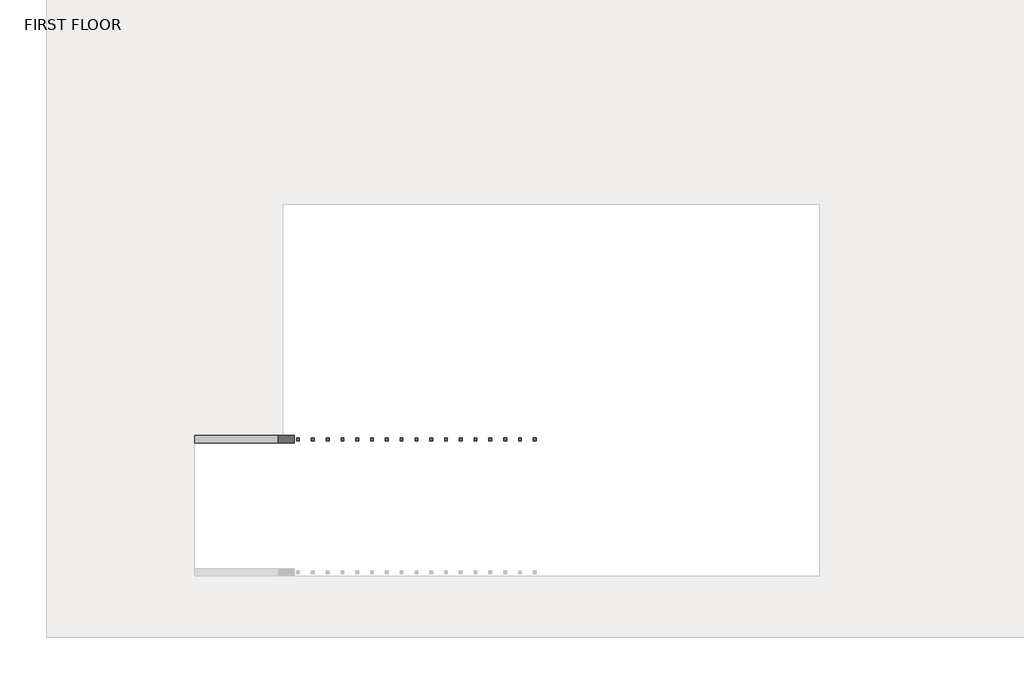
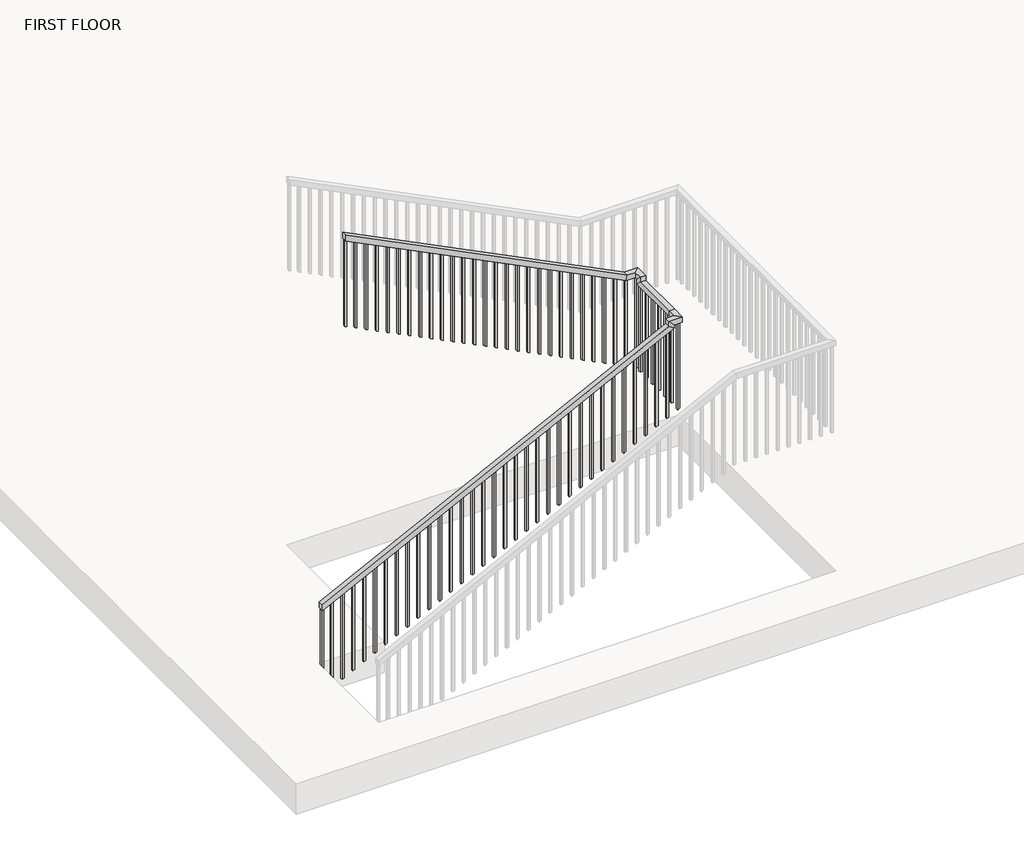
# One storey, part 2 of 2: 1 railing.
"""IFC4 building model written with IfcOpenShell, lengths in millimetres."""

from ifc_helpers import new_model, si_unit, frame, origin, place, context, project, spatial, polyline, outline, extrude, faceted_brep, element, save

model = new_model("IFC4")

# Units and contexts
model_context = context("Model", 3, world=origin())
ifc_project = project(units=[si_unit("LENGTHUNIT", "METRE", prefix="MILLI")], contexts=[model_context])

# Site, building, storey
site = spatial("IfcSite", under=ifc_project)
building = spatial("IfcBuilding", under=site)
storey = spatial("IfcBuildingStorey", under=building, Name="FIRST FLOOR", Elevation=3048.0)

# Railing
placement = place(None, origin())
element("IfcRailing", 1, ObjectType="Handrail - Rectangular", at=placement, inside=storey, context=model_context, shape_type="SolidModel", body=[
    faceted_brep([(-8362.2800418, -4455.7090076, 3962.4), (-8362.2800418, -4455.7090076, 3905.6038734), (-8362.2800418, -4506.5090076, 3905.6038734), (-8362.2800418, -4506.5090076, 3962.4), (-5111.0800418, -4455.7090076, 5588.0), (-5060.2800418, -4455.7090076, 5556.6038734), (-5060.2800418, -4506.5090076, 5556.6038734), (-5111.0800418, -4506.5090076, 5588.0), (-5111.0800418, -4455.7090076, 5638.8), (-5060.2800418, -4455.7090076, 5588.0), (-5060.2800418, -4506.5090076, 5588.0), (-5111.0800418, -4506.5090076, 5638.8), (-5034.8800418, -4455.7090076, 5638.8), (-5034.8800418, -4455.7090076, 5588.0), (-4984.0800418, -4506.5090076, 5588.0), (-4984.0800418, -4506.5090076, 5638.8), (-5034.8800418, -4379.5090076, 5638.8), (-5034.8800418, -4379.5090076, 5588.0), (-4984.0800418, -4379.5090076, 5588.0), (-4984.0800418, -4379.5090076, 5638.8), (-5034.8800418, -3907.7346494, 5638.8), (-5034.8800418, -3856.9346494, 5588.0), (-4984.0800418, -3856.9346494, 5588.0), (-4984.0800418, -3907.7346494, 5638.8), (-5034.8800418, -3907.7346494, 5689.6), (-5034.8800418, -3856.9346494, 5638.8), (-4984.0800418, -3856.9346494, 5638.8), (-4984.0800418, -3907.7346494, 5689.6), (-5034.8800418, -3831.5346494, 5689.6), (-5034.8800418, -3831.5346494, 5638.8), (-4984.0800418, -3780.7346494, 5638.8), (-4984.0800418, -3780.7346494, 5689.6), (-5111.0800418, -3831.5346494, 5689.6), (-5123.072295, -3831.5346494, 5638.8), (-5123.072295, -3780.7346494, 5638.8), (-5111.0800418, -3780.7346494, 5689.6), (-7752.6800418, -3831.5346494, 7010.4), (-7752.6800418, -3780.7346494, 7010.4), (-7752.6800418, -3780.7346494, 6953.6038734), (-7752.6800418, -3831.5346494, 6953.6038734)], [[[0, 1, 2, 3]], [[1, 0, 4, 5]], [[2, 1, 5, 6]], [[3, 2, 6, 7]], [[0, 3, 7, 4]], [[5, 4, 8, 9]], [[6, 5, 9, 10]], [[7, 6, 10, 11]], [[4, 7, 11, 8]], [[9, 8, 12, 13]], [[10, 9, 13, 14]], [[11, 10, 14, 15]], [[8, 11, 15, 12]], [[13, 12, 16, 17]], [[14, 13, 17, 18]], [[15, 14, 18, 19]], [[12, 15, 19, 16]], [[17, 16, 20, 21]], [[18, 17, 21, 22]], [[19, 18, 22, 23]], [[16, 19, 23, 20]], [[21, 20, 24, 25]], [[22, 21, 25, 26]], [[23, 22, 26, 27]], [[20, 23, 27, 24]], [[25, 24, 28, 29]], [[26, 25, 29, 30]], [[27, 26, 30, 31]], [[24, 27, 31, 28]], [[29, 28, 32, 33]], [[30, 29, 33, 34]], [[31, 30, 34, 35]], [[28, 31, 35, 32]], [[36, 37, 38, 39]], [[33, 32, 36, 39]], [[34, 33, 39, 38]], [[35, 34, 38, 37]], [[32, 35, 37, 36]]]),
    extrude(outline(polyline([(6898.0413734, -7641.5550418), (6907.5663734, -7660.6050418), (6049.9625, -7660.6050418), (6040.4375, -7641.5550418), (6898.0413734, -7641.5550418)])), frame((0.0, -3815.6596494, 0.0), z_axis=(0.0, 1.0, 0.0), x_axis=(0.0, 0.0, 1.0)), (0.0, 0.0, 1.0), 19.05),
    extrude(outline(polyline([(6847.2413734, -7539.9550418), (6856.7663734, -7559.0050418), (5999.1625, -7559.0050418), (5989.6375, -7539.9550418), (6847.2413734, -7539.9550418)])), frame((0.0, -3815.6596494, 0.0), z_axis=(0.0, 1.0, 0.0), x_axis=(0.0, 0.0, 1.0)), (0.0, 0.0, 1.0), 19.05),
    extrude(outline(polyline([(6796.4413734, -7438.3550418), (6805.9663734, -7457.4050418), (5948.3625, -7457.4050418), (5938.8375, -7438.3550418), (6796.4413734, -7438.3550418)])), frame((0.0, -3815.6596494, 0.0), z_axis=(0.0, 1.0, 0.0), x_axis=(0.0, 0.0, 1.0)), (0.0, 0.0, 1.0), 19.05),
    extrude(outline(polyline([(6745.6413734, -7336.7550418), (6755.1663734, -7355.8050418), (5897.5625, -7355.8050418), (5888.0375, -7336.7550418), (6745.6413734, -7336.7550418)])), frame((0.0, -3815.6596494, 0.0), z_axis=(0.0, 1.0, 0.0), x_axis=(0.0, 0.0, 1.0)), (0.0, 0.0, 1.0), 19.05),
    extrude(outline(polyline([(6694.8413734, -7235.1550418), (6704.3663734, -7254.2050418), (5846.7625, -7254.2050418), (5837.2375, -7235.1550418), (6694.8413734, -7235.1550418)])), frame((0.0, -3815.6596494, 0.0), z_axis=(0.0, 1.0, 0.0), x_axis=(0.0, 0.0, 1.0)), (0.0, 0.0, 1.0), 19.05),
    extrude(outline(polyline([(6644.0413734, -7133.5550418), (6653.5663734, -7152.6050418), (5795.9625, -7152.6050418), (5786.4375, -7133.5550418), (6644.0413734, -7133.5550418)])), frame((0.0, -3815.6596494, 0.0), z_axis=(0.0, 1.0, 0.0), x_axis=(0.0, 0.0, 1.0)), (0.0, 0.0, 1.0), 19.05),
    extrude(outline(polyline([(6593.2413734, -7031.9550418), (6602.7663734, -7051.0050418), (5745.1625, -7051.0050418), (5735.6375, -7031.9550418), (6593.2413734, -7031.9550418)])), frame((0.0, -3815.6596494, 0.0), z_axis=(0.0, 1.0, 0.0), x_axis=(0.0, 0.0, 1.0)), (0.0, 0.0, 1.0), 19.05),
    extrude(outline(polyline([(6542.4413734, -6930.3550418), (6551.9663734, -6949.4050418), (5694.3625, -6949.4050418), (5684.8375, -6930.3550418), (6542.4413734, -6930.3550418)])), frame((0.0, -3815.6596494, 0.0), z_axis=(0.0, 1.0, 0.0), x_axis=(0.0, 0.0, 1.0)), (0.0, 0.0, 1.0), 19.05),
    extrude(outline(polyline([(6491.6413734, -6828.7550418), (6501.1663734, -6847.8050418), (5643.5625, -6847.8050418), (5634.0375, -6828.7550418), (6491.6413734, -6828.7550418)])), frame((0.0, -3815.6596494, 0.0), z_axis=(0.0, 1.0, 0.0), x_axis=(0.0, 0.0, 1.0)), (0.0, 0.0, 1.0), 19.05),
    extrude(outline(polyline([(6440.8413734, -6727.1550418), (6450.3663734, -6746.2050418), (5592.7625, -6746.2050418), (5583.2375, -6727.1550418), (6440.8413734, -6727.1550418)])), frame((0.0, -3815.6596494, 0.0), z_axis=(0.0, 1.0, 0.0), x_axis=(0.0, 0.0, 1.0)), (0.0, 0.0, 1.0), 19.05),
    extrude(outline(polyline([(6390.0413734, -6625.5550418), (6399.5663734, -6644.6050418), (5541.9625, -6644.6050418), (5532.4375, -6625.5550418), (6390.0413734, -6625.5550418)])), frame((0.0, -3815.6596494, 0.0), z_axis=(0.0, 1.0, 0.0), x_axis=(0.0, 0.0, 1.0)), (0.0, 0.0, 1.0), 19.05),
    extrude(outline(polyline([(6339.2413734, -6523.9550418), (6348.7663734, -6543.0050418), (5491.1625, -6543.0050418), (5481.6375, -6523.9550418), (6339.2413734, -6523.9550418)])), frame((0.0, -3815.6596494, 0.0), z_axis=(0.0, 1.0, 0.0), x_axis=(0.0, 0.0, 1.0)), (0.0, 0.0, 1.0), 19.05),
    extrude(outline(polyline([(6288.4413734, -6422.3550418), (6297.9663734, -6441.4050418), (5440.3625, -6441.4050418), (5430.8375, -6422.3550418), (6288.4413734, -6422.3550418)])), frame((0.0, -3815.6596494, 0.0), z_axis=(0.0, 1.0, 0.0), x_axis=(0.0, 0.0, 1.0)), (0.0, 0.0, 1.0), 19.05),
    extrude(outline(polyline([(6237.6413734, -6320.7550418), (6247.1663734, -6339.8050418), (5389.5625, -6339.8050418), (5380.0375, -6320.7550418), (6237.6413734, -6320.7550418)])), frame((0.0, -3815.6596494, 0.0), z_axis=(0.0, 1.0, 0.0), x_axis=(0.0, 0.0, 1.0)), (0.0, 0.0, 1.0), 19.05),
    extrude(outline(polyline([(6186.8413734, -6219.1550418), (6196.3663734, -6238.2050418), (5338.7625, -6238.2050418), (5329.2375, -6219.1550418), (6186.8413734, -6219.1550418)])), frame((0.0, -3815.6596494, 0.0), z_axis=(0.0, 1.0, 0.0), x_axis=(0.0, 0.0, 1.0)), (0.0, 0.0, 1.0), 19.05),
    extrude(outline(polyline([(6136.0413734, -6117.5550418), (6145.5663734, -6136.6050418), (5287.9625, -6136.6050418), (5278.4375, -6117.5550418), (6136.0413734, -6117.5550418)])), frame((0.0, -3815.6596494, 0.0), z_axis=(0.0, 1.0, 0.0), x_axis=(0.0, 0.0, 1.0)), (0.0, 0.0, 1.0), 19.05),
    extrude(outline(polyline([(6085.2413734, -6015.9550418), (6094.7663734, -6035.0050418), (5237.1625, -6035.0050418), (5227.6375, -6015.9550418), (6085.2413734, -6015.9550418)])), frame((0.0, -3815.6596494, 0.0), z_axis=(0.0, 1.0, 0.0), x_axis=(0.0, 0.0, 1.0)), (0.0, 0.0, 1.0), 19.05),
    extrude(outline(polyline([(6034.4413734, -5914.3550418), (6043.9663734, -5933.4050418), (5186.3625, -5933.4050418), (5176.8375, -5914.3550418), (6034.4413734, -5914.3550418)])), frame((0.0, -3815.6596494, 0.0), z_axis=(0.0, 1.0, 0.0), x_axis=(0.0, 0.0, 1.0)), (0.0, 0.0, 1.0), 19.05),
    extrude(outline(polyline([(5983.6413734, -5812.7550418), (5993.1663734, -5831.8050418), (5135.5625, -5831.8050418), (5126.0375, -5812.7550418), (5983.6413734, -5812.7550418)])), frame((0.0, -3815.6596494, 0.0), z_axis=(0.0, 1.0, 0.0), x_axis=(0.0, 0.0, 1.0)), (0.0, 0.0, 1.0), 19.05),
    extrude(outline(polyline([(5932.8413734, -5711.1550418), (5942.3663734, -5730.2050418), (5084.7625, -5730.2050418), (5075.2375, -5711.1550418), (5932.8413734, -5711.1550418)])), frame((0.0, -3815.6596494, 0.0), z_axis=(0.0, 1.0, 0.0), x_axis=(0.0, 0.0, 1.0)), (0.0, 0.0, 1.0), 19.05),
    extrude(outline(polyline([(5882.0413734, -5609.5550418), (5891.5663734, -5628.6050418), (5033.9625, -5628.6050418), (5024.4375, -5609.5550418), (5882.0413734, -5609.5550418)])), frame((0.0, -3815.6596494, 0.0), z_axis=(0.0, 1.0, 0.0), x_axis=(0.0, 0.0, 1.0)), (0.0, 0.0, 1.0), 19.05),
    extrude(outline(polyline([(5831.2413734, -5507.9550418), (5840.7663734, -5527.0050418), (4983.1625, -5527.0050418), (4973.6375, -5507.9550418), (5831.2413734, -5507.9550418)])), frame((0.0, -3815.6596494, 0.0), z_axis=(0.0, 1.0, 0.0), x_axis=(0.0, 0.0, 1.0)), (0.0, 0.0, 1.0), 19.05),
    extrude(outline(polyline([(5780.4413734, -5406.3550418), (5789.9663734, -5425.4050418), (4932.3625, -5425.4050418), (4922.8375, -5406.3550418), (5780.4413734, -5406.3550418)])), frame((0.0, -3815.6596494, 0.0), z_axis=(0.0, 1.0, 0.0), x_axis=(0.0, 0.0, 1.0)), (0.0, 0.0, 1.0), 19.05),
    extrude(outline(polyline([(5729.6413734, -5304.7550418), (5739.1663734, -5323.8050418), (4881.5625, -5323.8050418), (4872.0375, -5304.7550418), (5729.6413734, -5304.7550418)])), frame((0.0, -3815.6596494, 0.0), z_axis=(0.0, 1.0, 0.0), x_axis=(0.0, 0.0, 1.0)), (0.0, 0.0, 1.0), 19.05),
    extrude(outline(polyline([(5678.8413734, -5203.1550418), (5688.3663734, -5222.2050418), (4830.7625, -5222.2050418), (4821.2375, -5203.1550418), (5678.8413734, -5203.1550418)])), frame((0.0, -3815.6596494, 0.0), z_axis=(0.0, 1.0, 0.0), x_axis=(0.0, 0.0, 1.0)), (0.0, 0.0, 1.0), 19.05),
    extrude(outline(polyline([(5638.8, -5101.5550418), (5638.8, -5120.6050418), (4779.9625, -5120.6050418), (4770.4375, -5101.5550418), (5638.8, -5101.5550418)])), frame((0.0, -3815.6596494, 0.0), z_axis=(0.0, 1.0, 0.0), x_axis=(0.0, 0.0, 1.0)), (0.0, 0.0, 1.0), 19.05),
    extrude(outline(polyline([(-4999.9550418, -3881.0340076), (-5019.0050418, -3881.0340076), (-5019.0050418, -3861.9840076), (-4999.9550418, -3861.9840076), (-4999.9550418, -3881.0340076)])), frame((0.0, 0.0, 4724.4), z_axis=(0.0, 0.0, 1.0), x_axis=(1.0, 0.0, 0.0)), (0.0, 0.0, 1.0), 863.6),
    extrude(outline(polyline([(-4999.9550418, -3982.6340076), (-5019.0050418, -3982.6340076), (-5019.0050418, -3963.5840076), (-4999.9550418, -3963.5840076), (-4999.9550418, -3982.6340076)])), frame((0.0, 0.0, 4724.4), z_axis=(0.0, 0.0, 1.0), x_axis=(1.0, 0.0, 0.0)), (0.0, 0.0, 1.0), 863.6),
    extrude(outline(polyline([(-4999.9550418, -4084.2340076), (-5019.0050418, -4084.2340076), (-5019.0050418, -4065.1840076), (-4999.9550418, -4065.1840076), (-4999.9550418, -4084.2340076)])), frame((0.0, 0.0, 4724.4), z_axis=(0.0, 0.0, 1.0), x_axis=(1.0, 0.0, 0.0)), (0.0, 0.0, 1.0), 863.6),
    extrude(outline(polyline([(-4999.9550418, -4185.8340076), (-5019.0050418, -4185.8340076), (-5019.0050418, -4166.7840076), (-4999.9550418, -4166.7840076), (-4999.9550418, -4185.8340076)])), frame((0.0, 0.0, 4724.4), z_axis=(0.0, 0.0, 1.0), x_axis=(1.0, 0.0, 0.0)), (0.0, 0.0, 1.0), 863.6),
    extrude(outline(polyline([(-4999.9550418, -4287.4340076), (-5019.0050418, -4287.4340076), (-5019.0050418, -4268.3840076), (-4999.9550418, -4268.3840076), (-4999.9550418, -4287.4340076)])), frame((0.0, 0.0, 4724.4), z_axis=(0.0, 0.0, 1.0), x_axis=(1.0, 0.0, 0.0)), (0.0, 0.0, 1.0), 863.6),
    extrude(outline(polyline([(-4999.9550418, -4389.0340076), (-5019.0050418, -4389.0340076), (-5019.0050418, -4369.9840076), (-4999.9550418, -4369.9840076), (-4999.9550418, -4389.0340076)])), frame((0.0, 0.0, 4724.4), z_axis=(0.0, 0.0, 1.0), x_axis=(1.0, 0.0, 0.0)), (0.0, 0.0, 1.0), 863.6),
    extrude(outline(polyline([(5535.9663734, -5101.5550418), (5526.4413734, -5120.6050418), (4668.8375, -5120.6050418), (4678.3625, -5101.5550418), (5535.9663734, -5101.5550418)])), frame((0.0, -4490.6340076, 0.0), z_axis=(0.0, 1.0, 0.0), x_axis=(0.0, 0.0, 1.0)), (0.0, 0.0, 1.0), 19.05),
    extrude(outline(polyline([(5485.1663734, -5203.1550418), (5475.6413734, -5222.2050418), (4618.0375, -5222.2050418), (4627.5625, -5203.1550418), (5485.1663734, -5203.1550418)])), frame((0.0, -4490.6340076, 0.0), z_axis=(0.0, 1.0, 0.0), x_axis=(0.0, 0.0, 1.0)), (0.0, 0.0, 1.0), 19.05),
    extrude(outline(polyline([(5434.3663734, -5304.7550418), (5424.8413734, -5323.8050418), (4567.2375, -5323.8050418), (4576.7625, -5304.7550418), (5434.3663734, -5304.7550418)])), frame((0.0, -4490.6340076, 0.0), z_axis=(0.0, 1.0, 0.0), x_axis=(0.0, 0.0, 1.0)), (0.0, 0.0, 1.0), 19.05),
    extrude(outline(polyline([(5383.5663734, -5406.3550418), (5374.0413734, -5425.4050418), (4516.4375, -5425.4050418), (4525.9625, -5406.3550418), (5383.5663734, -5406.3550418)])), frame((0.0, -4490.6340076, 0.0), z_axis=(0.0, 1.0, 0.0), x_axis=(0.0, 0.0, 1.0)), (0.0, 0.0, 1.0), 19.05),
    extrude(outline(polyline([(5332.7663734, -5507.9550418), (5323.2413734, -5527.0050418), (4465.6375, -5527.0050418), (4475.1625, -5507.9550418), (5332.7663734, -5507.9550418)])), frame((0.0, -4490.6340076, 0.0), z_axis=(0.0, 1.0, 0.0), x_axis=(0.0, 0.0, 1.0)), (0.0, 0.0, 1.0), 19.05),
    extrude(outline(polyline([(5281.9663734, -5609.5550418), (5272.4413734, -5628.6050418), (4414.8375, -5628.6050418), (4424.3625, -5609.5550418), (5281.9663734, -5609.5550418)])), frame((0.0, -4490.6340076, 0.0), z_axis=(0.0, 1.0, 0.0), x_axis=(0.0, 0.0, 1.0)), (0.0, 0.0, 1.0), 19.05),
    extrude(outline(polyline([(5231.1663734, -5711.1550418), (5221.6413734, -5730.2050418), (4364.0375, -5730.2050418), (4373.5625, -5711.1550418), (5231.1663734, -5711.1550418)])), frame((0.0, -4490.6340076, 0.0), z_axis=(0.0, 1.0, 0.0), x_axis=(0.0, 0.0, 1.0)), (0.0, 0.0, 1.0), 19.05),
    extrude(outline(polyline([(5180.3663734, -5812.7550418), (5170.8413734, -5831.8050418), (4313.2375, -5831.8050418), (4322.7625, -5812.7550418), (5180.3663734, -5812.7550418)])), frame((0.0, -4490.6340076, 0.0), z_axis=(0.0, 1.0, 0.0), x_axis=(0.0, 0.0, 1.0)), (0.0, 0.0, 1.0), 19.05),
    extrude(outline(polyline([(5129.5663734, -5914.3550418), (5120.0413734, -5933.4050418), (4262.4375, -5933.4050418), (4271.9625, -5914.3550418), (5129.5663734, -5914.3550418)])), frame((0.0, -4490.6340076, 0.0), z_axis=(0.0, 1.0, 0.0), x_axis=(0.0, 0.0, 1.0)), (0.0, 0.0, 1.0), 19.05),
    extrude(outline(polyline([(5078.7663734, -6015.9550418), (5069.2413734, -6035.0050418), (4211.6375, -6035.0050418), (4221.1625, -6015.9550418), (5078.7663734, -6015.9550418)])), frame((0.0, -4490.6340076, 0.0), z_axis=(0.0, 1.0, 0.0), x_axis=(0.0, 0.0, 1.0)), (0.0, 0.0, 1.0), 19.05),
    extrude(outline(polyline([(5027.9663734, -6117.5550418), (5018.4413734, -6136.6050418), (4160.8375, -6136.6050418), (4170.3625, -6117.5550418), (5027.9663734, -6117.5550418)])), frame((0.0, -4490.6340076, 0.0), z_axis=(0.0, 1.0, 0.0), x_axis=(0.0, 0.0, 1.0)), (0.0, 0.0, 1.0), 19.05),
    extrude(outline(polyline([(4977.1663734, -6219.1550418), (4967.6413734, -6238.2050418), (4110.0375, -6238.2050418), (4119.5625, -6219.1550418), (4977.1663734, -6219.1550418)])), frame((0.0, -4490.6340076, 0.0), z_axis=(0.0, 1.0, 0.0), x_axis=(0.0, 0.0, 1.0)), (0.0, 0.0, 1.0), 19.05),
    extrude(outline(polyline([(4926.3663734, -6320.7550418), (4916.8413734, -6339.8050418), (4059.2375, -6339.8050418), (4068.7625, -6320.7550418), (4926.3663734, -6320.7550418)])), frame((0.0, -4490.6340076, 0.0), z_axis=(0.0, 1.0, 0.0), x_axis=(0.0, 0.0, 1.0)), (0.0, 0.0, 1.0), 19.05),
    extrude(outline(polyline([(4875.5663734, -6422.3550418), (4866.0413734, -6441.4050418), (4008.4375, -6441.4050418), (4017.9625, -6422.3550418), (4875.5663734, -6422.3550418)])), frame((0.0, -4490.6340076, 0.0), z_axis=(0.0, 1.0, 0.0), x_axis=(0.0, 0.0, 1.0)), (0.0, 0.0, 1.0), 19.05),
    extrude(outline(polyline([(4824.7663734, -6523.9550418), (4815.2413734, -6543.0050418), (3957.6375, -6543.0050418), (3967.1625, -6523.9550418), (4824.7663734, -6523.9550418)])), frame((0.0, -4490.6340076, 0.0), z_axis=(0.0, 1.0, 0.0), x_axis=(0.0, 0.0, 1.0)), (0.0, 0.0, 1.0), 19.05),
    extrude(outline(polyline([(4773.9663734, -6625.5550418), (4764.4413734, -6644.6050418), (3906.8375, -6644.6050418), (3916.3625, -6625.5550418), (4773.9663734, -6625.5550418)])), frame((0.0, -4490.6340076, 0.0), z_axis=(0.0, 1.0, 0.0), x_axis=(0.0, 0.0, 1.0)), (0.0, 0.0, 1.0), 19.05),
    extrude(outline(polyline([(4723.1663734, -6727.1550418), (4713.6413734, -6746.2050418), (3856.0375, -6746.2050418), (3865.5625, -6727.1550418), (4723.1663734, -6727.1550418)])), frame((0.0, -4490.6340076, 0.0), z_axis=(0.0, 1.0, 0.0), x_axis=(0.0, 0.0, 1.0)), (0.0, 0.0, 1.0), 19.05),
    extrude(outline(polyline([(4672.3663734, -6828.7550418), (4662.8413734, -6847.8050418), (3805.2375, -6847.8050418), (3814.7625, -6828.7550418), (4672.3663734, -6828.7550418)])), frame((0.0, -4490.6340076, 0.0), z_axis=(0.0, 1.0, 0.0), x_axis=(0.0, 0.0, 1.0)), (0.0, 0.0, 1.0), 19.05),
    extrude(outline(polyline([(4621.5663734, -6930.3550418), (4612.0413734, -6949.4050418), (3754.4375, -6949.4050418), (3763.9625, -6930.3550418), (4621.5663734, -6930.3550418)])), frame((0.0, -4490.6340076, 0.0), z_axis=(0.0, 1.0, 0.0), x_axis=(0.0, 0.0, 1.0)), (0.0, 0.0, 1.0), 19.05),
    extrude(outline(polyline([(4570.7663734, -7031.9550418), (4561.2413734, -7051.0050418), (3703.6375, -7051.0050418), (3713.1625, -7031.9550418), (4570.7663734, -7031.9550418)])), frame((0.0, -4490.6340076, 0.0), z_axis=(0.0, 1.0, 0.0), x_axis=(0.0, 0.0, 1.0)), (0.0, 0.0, 1.0), 19.05),
    extrude(outline(polyline([(4519.9663734, -7133.5550418), (4510.4413734, -7152.6050418), (3652.8375, -7152.6050418), (3662.3625, -7133.5550418), (4519.9663734, -7133.5550418)])), frame((0.0, -4490.6340076, 0.0), z_axis=(0.0, 1.0, 0.0), x_axis=(0.0, 0.0, 1.0)), (0.0, 0.0, 1.0), 19.05),
    extrude(outline(polyline([(4469.1663734, -7235.1550418), (4459.6413734, -7254.2050418), (3602.0375, -7254.2050418), (3611.5625, -7235.1550418), (4469.1663734, -7235.1550418)])), frame((0.0, -4490.6340076, 0.0), z_axis=(0.0, 1.0, 0.0), x_axis=(0.0, 0.0, 1.0)), (0.0, 0.0, 1.0), 19.05),
    extrude(outline(polyline([(4418.3663734, -7336.7550418), (4408.8413734, -7355.8050418), (3551.2375, -7355.8050418), (3560.7625, -7336.7550418), (4418.3663734, -7336.7550418)])), frame((0.0, -4490.6340076, 0.0), z_axis=(0.0, 1.0, 0.0), x_axis=(0.0, 0.0, 1.0)), (0.0, 0.0, 1.0), 19.05),
    extrude(outline(polyline([(4367.5663734, -7438.3550418), (4358.0413734, -7457.4050418), (3500.4375, -7457.4050418), (3509.9625, -7438.3550418), (4367.5663734, -7438.3550418)])), frame((0.0, -4490.6340076, 0.0), z_axis=(0.0, 1.0, 0.0), x_axis=(0.0, 0.0, 1.0)), (0.0, 0.0, 1.0), 19.05),
    extrude(outline(polyline([(4316.7663734, -7539.9550418), (4307.2413734, -7559.0050418), (3449.6375, -7559.0050418), (3459.1625, -7539.9550418), (4316.7663734, -7539.9550418)])), frame((0.0, -4490.6340076, 0.0), z_axis=(0.0, 1.0, 0.0), x_axis=(0.0, 0.0, 1.0)), (0.0, 0.0, 1.0), 19.05),
    extrude(outline(polyline([(4265.9663734, -7641.5550418), (4256.4413734, -7660.6050418), (3398.8375, -7660.6050418), (3408.3625, -7641.5550418), (4265.9663734, -7641.5550418)])), frame((0.0, -4490.6340076, 0.0), z_axis=(0.0, 1.0, 0.0), x_axis=(0.0, 0.0, 1.0)), (0.0, 0.0, 1.0), 19.05),
    extrude(outline(polyline([(4215.1663734, -7743.1550418), (4205.6413734, -7762.2050418), (3348.0375, -7762.2050418), (3357.5625, -7743.1550418), (4215.1663734, -7743.1550418)])), frame((0.0, -4490.6340076, 0.0), z_axis=(0.0, 1.0, 0.0), x_axis=(0.0, 0.0, 1.0)), (0.0, 0.0, 1.0), 19.05),
    extrude(outline(polyline([(4164.3663734, -7844.7550418), (4154.8413734, -7863.8050418), (3297.2375, -7863.8050418), (3306.7625, -7844.7550418), (4164.3663734, -7844.7550418)])), frame((0.0, -4490.6340076, 0.0), z_axis=(0.0, 1.0, 0.0), x_axis=(0.0, 0.0, 1.0)), (0.0, 0.0, 1.0), 19.05),
    extrude(outline(polyline([(4113.5663734, -7946.3550418), (4104.0413734, -7965.4050418), (3246.4375, -7965.4050418), (3255.9625, -7946.3550418), (4113.5663734, -7946.3550418)])), frame((0.0, -4490.6340076, 0.0), z_axis=(0.0, 1.0, 0.0), x_axis=(0.0, 0.0, 1.0)), (0.0, 0.0, 1.0), 19.05),
    extrude(outline(polyline([(4062.7663734, -8047.9550418), (4053.2413734, -8067.0050418), (3195.6375, -8067.0050418), (3205.1625, -8047.9550418), (4062.7663734, -8047.9550418)])), frame((0.0, -4490.6340076, 0.0), z_axis=(0.0, 1.0, 0.0), x_axis=(0.0, 0.0, 1.0)), (0.0, 0.0, 1.0), 19.05),
    extrude(outline(polyline([(4011.9663734, -8149.5550418), (4002.4413734, -8168.6050418), (3144.8375, -8168.6050418), (3154.3625, -8149.5550418), (4011.9663734, -8149.5550418)])), frame((0.0, -4490.6340076, 0.0), z_axis=(0.0, 1.0, 0.0), x_axis=(0.0, 0.0, 1.0)), (0.0, 0.0, 1.0), 19.05),
    extrude(outline(polyline([(3961.1663734, -8251.1550418), (3951.6413734, -8270.2050418), (3094.0375, -8270.2050418), (3103.5625, -8251.1550418), (3961.1663734, -8251.1550418)])), frame((0.0, -4490.6340076, 0.0), z_axis=(0.0, 1.0, 0.0), x_axis=(0.0, 0.0, 1.0)), (0.0, 0.0, 1.0), 19.05),
    extrude(outline(polyline([(-4999.9550418, -3815.6596494), (-5019.0050418, -3815.6596494), (-5019.0050418, -3796.6096494), (-4999.9550418, -3796.6096494), (-4999.9550418, -3815.6596494)])), frame((0.0, 0.0, 4724.4), z_axis=(0.0, 0.0, 1.0), x_axis=(1.0, 0.0, 0.0)), (0.0, 0.0, 1.0), 914.4),
    extrude(outline(polyline([(5588.0, -4999.9550418), (5588.0, -5019.0050418), (4719.6375, -5019.0050418), (4729.1625, -4999.9550418), (5588.0, -4999.9550418)])), frame((0.0, -4490.6340076, 0.0), z_axis=(0.0, 1.0, 0.0), x_axis=(0.0, 0.0, 1.0)), (0.0, 0.0, 1.0), 19.05),
    extrude(outline(polyline([(6944.0788734, -7733.6300418), (6953.6038734, -7752.6800418), (6096.0, -7752.6800418), (6086.475, -7733.6300418), (6944.0788734, -7733.6300418)])), frame((0.0, -3815.6596494, 0.0), z_axis=(0.0, 1.0, 0.0), x_axis=(0.0, 0.0, 1.0)), (0.0, 0.0, 1.0), 19.05),
    extrude(outline(polyline([(3915.1288734, -8343.2300418), (3905.6038734, -8362.2800418), (3048.0, -8362.2800418), (3057.525, -8343.2300418), (3915.1288734, -8343.2300418)])), frame((0.0, -4490.6340076, 0.0), z_axis=(0.0, 1.0, 0.0), x_axis=(0.0, 0.0, 1.0)), (0.0, 0.0, 1.0), 19.05),
])

save(model, "model.ifc")

# Revit data of these elements
# Type "Handrail - Rectangular"
#   Assembly Code = "C2010400"
#   built-in parameter 1008612 = 0.0416667 (stored number, unit not read)
#   built-in parameter 1008611 = 0.0416667 (stored number, unit not read)
#   built-in parameter 1008609 = 0.333333 (stored number, unit not read)
#   built-in parameter 1008604 = 0.166667 (stored number, unit not read)
#   built-in parameter 1008603 = 0.166667 (stored number, unit not read)
#   Railing Height = 3' - 0"
#   built-in parameter 1008630 = 2
#   built-in parameter 1008610 = 2
#   built-in parameter 1008618 = Baluster - Square : 3/4"
# Element 1 (IfcRailing, "Handrail - Rectangular")
#   Phase Created = New Construction
